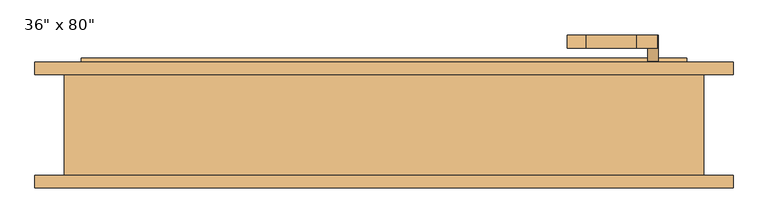
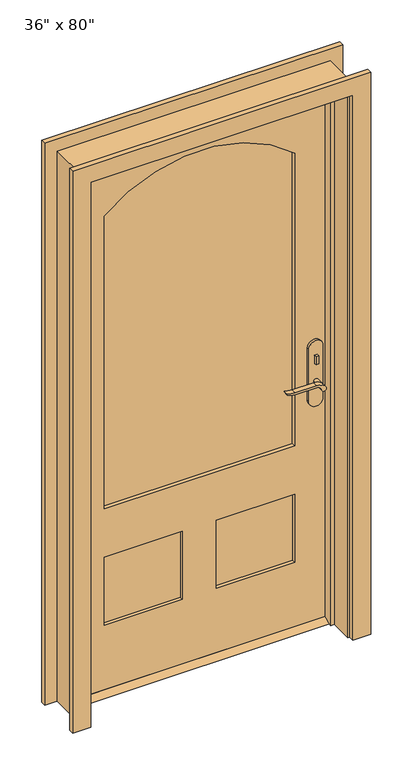
"""IFC4 building model written with IfcOpenShell, lengths in millimetres: door geometry."""

from ifc_helpers import new_model, si_unit, point, frame, frame_2d, origin, place, context, project, spatial, polyline, circle_curve, trimmed, segment, composite_curve, outline, extrude, faceted_brep, source, transform, mapped, element, save


def door_808aeb8e(model_context):
    return source(origin(), model_context, "Body", "SolidModel", [
        extrude(outline(polyline([(38.1, 12.7), (73.025, 12.7), (98.425, 0.0), (12.7, 0.0), (38.1, 12.7)])), frame((-457.2, 0.0, 0.0), z_axis=(1.0, 0.0, 0.0), x_axis=(0.0, 1.0, 0.0)), (0.0, 0.0, 1.0), 914.4),
        extrude(outline(polyline([(411.4, 18.1), (401.4, 18.1), (401.4, 28.1), (411.4, 28.1), (411.4, 18.1)])), frame((0.0, 0.0, 981.9), z_axis=(0.0, 0.0, 1.0), x_axis=(1.0, 0.0, 0.0)), (0.0, 0.0, 1.0), 30.0),
        extrude(outline(composite_curve([segment(trimmed(circle_curve(frame_2d((996.9, 406.4)), 8.0), [point((996.9, 398.4))], [point((996.9, 414.4))], False, "CARTESIAN"), True, "CONTINUOUS"), segment(trimmed(circle_curve(frame_2d((996.9, 406.4)), 8.0), [point((996.9, 414.4))], [point((996.9, 398.4))], False, "CARTESIAN"), True, "CONTINUOUS")], self_intersect=False)), frame((0.0, 83.025, 0.0), z_axis=(0.0, 1.0, 0.0), x_axis=(0.0, 0.0, 1.0)), (0.0, 0.0, 1.0), 10.0),
        extrude(outline(composite_curve([segment(trimmed(circle_curve(frame_2d((897.1555521, 382.7324871)), 37.2832219), [point((919.0523287, 412.9081363))], [point((934.4, 381.0325667))], False, "CARTESIAN"), True, "CONTINUOUS"), segment(polyline([(934.4, 381.0325667), (934.4, 304.7564091)]), True, "CONTINUOUS"), segment(trimmed(circle_curve(frame_2d((1017.6850638, 304.8227909)), 83.2850902), [point((934.4, 304.7564091))], [point((939.4, 276.4))], True, "CARTESIAN"), True, "CONTINUOUS"), segment(polyline([(939.4, 276.4), (936.6135558, 276.4)]), True, "CONTINUOUS"), segment(trimmed(circle_curve(frame_2d((986.6709207, 308.3396612)), 59.3791355), [point((936.6135558, 276.4))], [point((927.4, 304.7564091))], False, "CARTESIAN"), True, "CONTINUOUS"), segment(polyline([(927.4, 304.7564091), (927.4, 381.0138099)]), True, "CONTINUOUS"), segment(trimmed(circle_curve(frame_2d((909.2738613, 381.0138099)), 18.1261387), [point((927.4, 381.0138099))], [point((914.4, 398.4))], True, "CARTESIAN"), True, "CONTINUOUS"), segment(trimmed(circle_curve(frame_2d((914.4, 406.4)), 8.0), [point((914.4, 398.4))], [point((919.0523287, 412.9081363))], False, "CARTESIAN"), True, "CONTINUOUS")], self_intersect=False)), frame((0.0, -21.9, 0.0), z_axis=(0.0, 1.0, 0.0), x_axis=(0.0, 0.0, 1.0)), (0.0, 0.0, 1.0), 20.0),
        extrude(outline(composite_curve([segment(trimmed(circle_curve(frame_2d((914.4, 406.4)), 8.0), [point((914.3999903, 398.4))], [point((919.0523287, 412.9081363))], False, "CARTESIAN"), True, "CONTINUOUS"), segment(trimmed(circle_curve(frame_2d((897.1555521, 382.7324871)), 37.2832219), [point((919.0523287, 412.9081363))], [point((934.4, 381.0325667))], False, "CARTESIAN"), True, "CONTINUOUS"), segment(polyline([(934.4, 381.0325667), (934.4, 304.7564091)]), True, "CONTINUOUS"), segment(trimmed(circle_curve(frame_2d((1017.6850638, 304.8227909)), 83.2850902), [point((934.4, 304.7564091))], [point((939.4, 276.4))], True, "CARTESIAN"), True, "CONTINUOUS"), segment(polyline([(939.4, 276.4), (936.6135558, 276.4)]), True, "CONTINUOUS"), segment(trimmed(circle_curve(frame_2d((986.6709207, 308.3396612)), 59.3791355), [point((936.6135558, 276.4))], [point((927.4, 304.7564091))], False, "CARTESIAN"), True, "CONTINUOUS"), segment(polyline([(927.4, 304.7564091), (927.4, 381.0138122)]), True, "CONTINUOUS"), segment(trimmed(circle_curve(frame_2d((909.2738682, 381.0138122)), 18.1261318), [point((927.4, 381.0138122))], [point((914.3999903, 398.4))], True, "CARTESIAN"), True, "CONTINUOUS")], self_intersect=False)), frame((0.0, 113.025, 0.0), z_axis=(0.0, 1.0, 0.0), x_axis=(0.0, 0.0, 1.0)), (0.0, 0.0, 1.0), 20.0),
        extrude(outline(composite_curve([segment(trimmed(circle_curve(frame_2d((914.4, 406.4)), 8.0), [point((914.4, 398.4))], [point((914.4, 414.4))], False, "CARTESIAN"), True, "CONTINUOUS"), segment(trimmed(circle_curve(frame_2d((914.4, 406.4)), 8.0), [point((914.4, 414.4))], [point((914.4, 398.4))], False, "CARTESIAN"), True, "CONTINUOUS")], self_intersect=False)), frame((0.0, -1.9, 0.0), z_axis=(0.0, 1.0, 0.0), x_axis=(0.0, 0.0, 1.0)), (0.0, 0.0, 1.0), 30.0),
        extrude(outline(composite_curve([segment(trimmed(circle_curve(frame_2d((914.4, 406.4)), 8.0), [point((914.4, 398.4))], [point((914.4, 414.4))], False, "CARTESIAN"), True, "CONTINUOUS"), segment(trimmed(circle_curve(frame_2d((914.4, 406.4)), 8.0), [point((914.4, 414.4))], [point((914.4, 398.4))], False, "CARTESIAN"), True, "CONTINUOUS")], self_intersect=False)), frame((0.0, 83.025, 0.0), z_axis=(0.0, 1.0, 0.0), x_axis=(0.0, 0.0, 1.0)), (0.0, 0.0, 1.0), 30.0),
        extrude(outline(composite_curve([segment(polyline([(844.4, 431.4), (1039.4, 431.4)]), True, "CONTINUOUS"), segment(trimmed(circle_curve(frame_2d((1039.4, 406.4)), 25.0), [point((1039.4, 431.4))], [point((1039.4, 381.4))], False, "CARTESIAN"), True, "CONTINUOUS"), segment(polyline([(1039.4, 381.4), (844.4, 381.4)]), True, "CONTINUOUS"), segment(trimmed(circle_curve(frame_2d((844.4, 406.4)), 25.0), [point((844.4, 381.4))], [point((844.4, 431.4))], False, "CARTESIAN"), True, "CONTINUOUS")], self_intersect=False)), frame((0.0, 28.1, 0.0), z_axis=(0.0, 1.0, 0.0), x_axis=(0.0, 0.0, 1.0)), (0.0, 0.0, 1.0), 10.0),
        extrude(outline(composite_curve([segment(polyline([(844.4, 431.4), (1039.4, 431.4)]), True, "CONTINUOUS"), segment(trimmed(circle_curve(frame_2d((1039.4, 406.4)), 25.0), [point((1039.4, 431.4))], [point((1039.4, 381.4))], False, "CARTESIAN"), True, "CONTINUOUS"), segment(polyline([(1039.4, 381.4), (844.4, 381.4)]), True, "CONTINUOUS"), segment(trimmed(circle_curve(frame_2d((844.4, 406.4)), 25.0), [point((844.4, 381.4))], [point((844.4, 431.4))], False, "CARTESIAN"), True, "CONTINUOUS")], self_intersect=False)), frame((0.0, 73.025, 0.0), z_axis=(0.0, 1.0, 0.0), x_axis=(0.0, 0.0, 1.0)), (0.0, 0.0, 1.0), 10.0),
        extrude(outline(polyline([(2032.0, -457.2), (12.7, -457.2), (12.7, 457.2), (2032.0, 457.2), (2032.0, -457.2)]), holes=[composite_curve([segment(polyline([(688.975, -336.55), (1784.35, -336.55)]), True, "CONTINUOUS"), segment(trimmed(circle_curve(frame_2d((1401.92125, 0.0)), 509.42875), [point((1784.35, -336.55))], [point((1784.35, 336.55))], True, "CARTESIAN"), True, "CONTINUOUS"), segment(polyline([(1784.35, 336.55), (688.975, 336.55), (688.975, -336.55)]), True, "CONTINUOUS")], self_intersect=False), polyline([(508.0, -60.325), (254.0, -60.325), (254.0, -336.55), (508.0, -336.55), (508.0, -60.325)]), polyline([(508.0, 336.55), (254.0, 336.55), (254.0, 60.325), (508.0, 60.325), (508.0, 336.55)])]), frame((0.0, 38.1, 0.0), z_axis=(0.0, 1.0, 0.0), x_axis=(0.0, 0.0, 1.0)), (0.0, 0.0, 1.0), 34.925),
        faceted_brep([(482.6, 73.025, 0.0), (482.6, -79.375, 0.0), (457.2, -79.375, 0.0), (457.2, 3.175, 0.0), (444.5, 3.175, 0.0), (444.5, 38.1, 0.0), (457.2, 38.1, 0.0), (457.2, 73.025, 0.0), (482.6, 73.025, 2057.4), (482.6, -79.375, 2057.4), (-482.6, -79.375, 2057.4), (-482.6, -79.375, 0.0), (-457.2, -79.375, 0.0), (-457.2, -79.375, 2032.0), (457.2, -79.375, 2032.0), (457.2, 3.175, 2032.0), (-457.2, 3.175, 2032.0), (-457.2, 3.175, 0.0), (-444.5, 3.175, 0.0), (-444.5, 3.175, 2019.3), (444.5, 3.175, 2019.3), (444.5, 38.1, 2019.3), (-444.5, 38.1, 2019.3), (-444.5, 38.1, 0.0), (-457.2, 38.1, 0.0), (-457.2, 38.1, 2032.0), (457.2, 38.1, 2032.0), (457.2, 73.025, 2032.0), (-457.2, 73.025, 2032.0), (-457.2, 73.025, 0.0), (-482.6, 73.025, 0.0), (-482.6, 73.025, 2057.4)], [[[0, 1, 2, 3, 4, 5, 6, 7]], [[1, 0, 8, 9]], [[2, 1, 9, 10, 11, 12, 13, 14]], [[3, 2, 14, 15]], [[4, 3, 15, 16, 17, 18, 19, 20]], [[5, 4, 20, 21]], [[6, 5, 21, 22, 23, 24, 25, 26]], [[7, 6, 26, 27]], [[0, 7, 27, 28, 29, 30, 31, 8]], [[9, 8, 31, 10]], [[15, 14, 13, 16]], [[21, 20, 19, 22]], [[27, 26, 25, 28]], [[30, 29, 24, 23, 18, 17, 12, 11]], [[10, 31, 30, 11]], [[16, 13, 12, 17]], [[22, 19, 18, 23]], [[28, 25, 24, 29]]]),
        extrude(outline(polyline([(-60.325, 49.7416667), (-336.55, 49.7416667), (-336.55, 61.3833333), (-60.325, 61.3833333), (-60.325, 49.7416667)])), frame((0.0, 0.0, 254.0), z_axis=(0.0, 0.0, 1.0), x_axis=(1.0, 0.0, 0.0)), (0.0, 0.0, 1.0), 254.0),
        extrude(outline(polyline([(336.55, 49.7416667), (60.325, 49.7416667), (60.325, 61.3833333), (336.55, 61.3833333), (336.55, 49.7416667)])), frame((0.0, 0.0, 254.0), z_axis=(0.0, 0.0, 1.0), x_axis=(1.0, 0.0, 0.0)), (0.0, 0.0, 1.0), 254.0),
        extrude(outline(composite_curve([segment(polyline([(688.975, -336.55), (688.975, 336.55), (1784.35, 336.55)]), True, "CONTINUOUS"), segment(trimmed(circle_curve(frame_2d((1401.92125, 0.0)), 509.42875), [point((1784.35, 336.55))], [point((1784.35, -336.55))], False, "CARTESIAN"), True, "CONTINUOUS"), segment(polyline([(1784.35, -336.55), (688.975, -336.55)]), True, "CONTINUOUS")], self_intersect=False)), frame((0.0, 52.07, 0.0), z_axis=(0.0, 1.0, 0.0), x_axis=(0.0, 0.0, 1.0)), (0.0, 0.0, 1.0), 6.985),
        extrude(outline(polyline([(0.0, -527.05), (0.0, -463.55), (2038.35, -463.55), (2038.35, 463.55), (0.0, 463.55), (0.0, 527.05), (2101.85, 527.05), (2101.85, -527.05), (0.0, -527.05)])), frame((0.0, -98.425, 0.0), z_axis=(0.0, 1.0, 0.0), x_axis=(0.0, 0.0, 1.0)), (0.0, 0.0, 1.0), 19.05),
        extrude(outline(polyline([(0.0, -527.05), (0.0, -463.55), (2038.35, -463.55), (2038.35, 463.55), (0.0, 463.55), (0.0, 527.05), (2101.85, 527.05), (2101.85, -527.05), (0.0, -527.05)])), frame((0.0, 73.025, 0.0), z_axis=(0.0, 1.0, 0.0), x_axis=(0.0, 0.0, 1.0)), (0.0, 0.0, 1.0), 19.05),
    ])


if __name__ == "__main__":
    model = new_model("IFC4")
    model_context = context("Model", 3, world=origin())
    ifc_project = project(units=[si_unit("LENGTHUNIT", "METRE", prefix="MILLI")], contexts=[model_context])
    site = spatial("IfcSite", under=ifc_project)
    building = spatial("IfcBuilding", under=site)
    placement = place(None, origin())
    door_shape = door_808aeb8e(model_context)
    element("IfcDoor", 1, ObjectType="36\" x 80\"", at=placement, inside=building, context=model_context, shape_type="MappedRepresentation", body=[
        mapped(door_shape, transform((0.0, 0.0, 0.0), x_axis=(1.0, 0.0, 0.0), y_axis=(0.0, 1.0, 0.0), z_axis=(0.0, 0.0, 1.0))),
    ])
    save(model, "model.ifc")

# Revit data of these elements
# Type "36\" x 80\""
#   Type Mark = "15"
#   Assembly Code = "B2030100"
#   Analytic Construction = "French door, wood frame with single glass"
#   Threshold Offset [instance default] = 0' - 0 1/2"
#   Thickness = 0' - 1 3/8"
#   Thermal Resistance (R) = 1.0696 (h·ft²·°F)/BTU
#   Swing Angle [instance default] = 90.00°
#   Stiles = 0' - 4 3/4"
#   Rough Width = 3' - 2"
#   Rough Height = 6' - 9"
#   Radius = 1' - 8.05625"
#   Lock Rail = 0' - 7 1/8"
#   Height = 6' - 8"
#   Width = 3' - 0"
#   Heat Transfer Coefficient (U) = 0.9350 BTU/(h·ft²·°F)
#   Door Offset [instance default] = 0' - 0"
#   Bottom Rail = 0' - 9 1/2"
#   Threshold [instance default] = yes
#   Function = 1
#   Exterior Trim [instance default] = yes
#   Trim Material = Cherry
#   Threshold Material = Cherry
#   Panel Material = Cherry
#   Glazing = Glass
#   Frame Material = Cherry
#   Door Handle Material = Aluminum
#   Visual Light Transmittance = 0
#   Solar Heat Gain Coefficient = 0
#   Wall Closure = (empty or 0)
#   Construction Type = (empty or 0)
# Element 1 (IfcDoor, "36\" x 80\"")
#   Materials on its faces: "Cherry", "Aluminum", "Glass"
# Materials
#   "Cherry": class "Wood", colour RGB 226 177 128, transparency 0, Description = "Prunus Serotina", Cost = 0
#   "Glass": class "Glass", colour RGB 0 128 192, transparency 0.75, Description = "Soda Lime Glass", Cost = 0
#   "Aluminum": class "Metal", colour RGB 247 247 247, transparency 0, Description = "Aluminum 6061", Cost = 0
